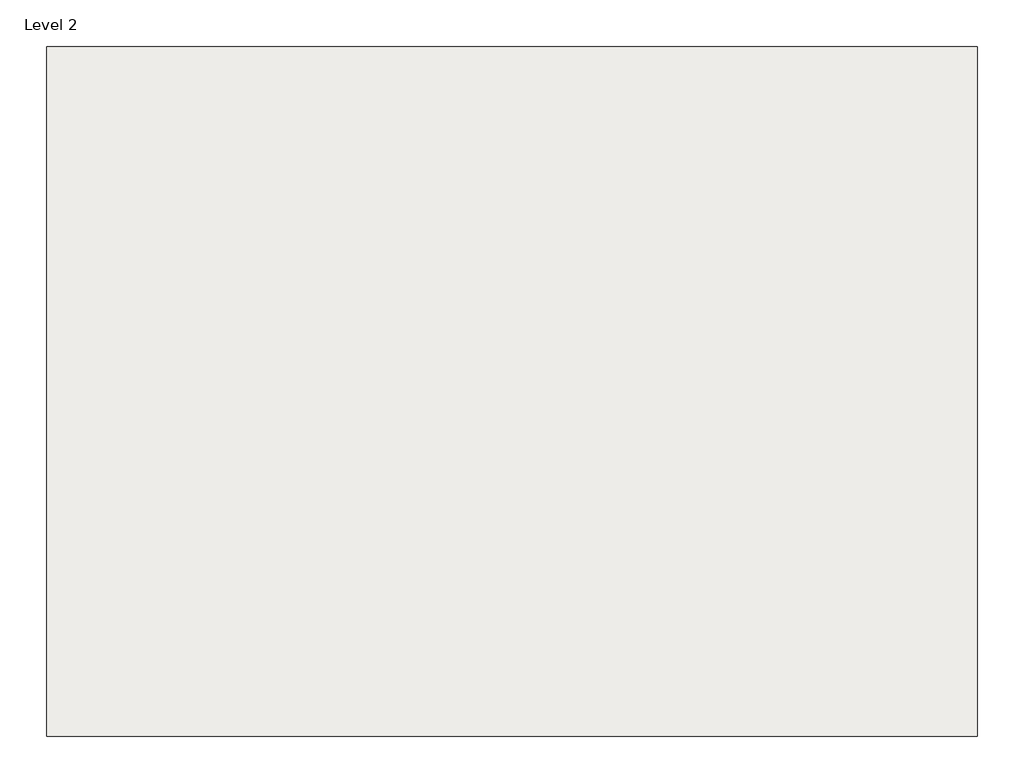
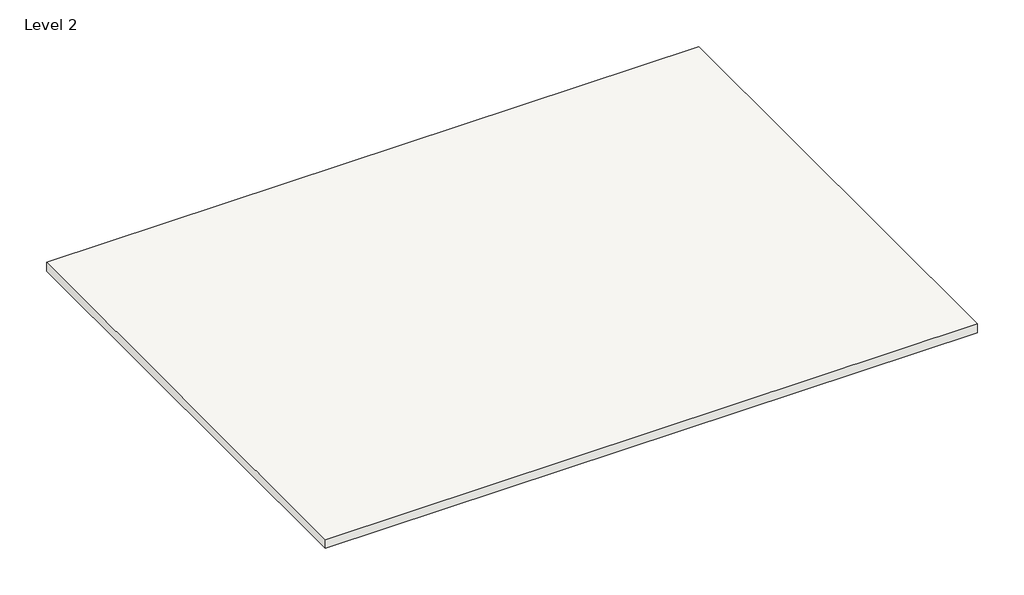
# One storey, incomplete: 1 roof.
"""IFC4 building model written with IfcOpenShell, lengths in millimetres."""

from ifc_helpers import new_model, si_unit, frame, origin, place, context, project, spatial, polyline, outline, extrude, element, save

model = new_model("IFC4")

# Units and contexts
model_context = context("Model", 3, world=origin())
ifc_project = project(units=[si_unit("LENGTHUNIT", "METRE", prefix="MILLI")], contexts=[model_context])

# Site, building, storey
site = spatial("IfcSite", under=ifc_project)
building = spatial("IfcBuilding", under=site)
storey = spatial("IfcBuildingStorey", under=building, Name="Level 2", Elevation=3048.0)

# Roof
placement = place(None, origin())
element("IfcRoof", 1, ObjectType="6\" floor", at=placement, inside=storey, context=model_context, shape_type="SweptSolid", body=[
    extrude(outline(polyline([(733.2620146, -5806.4506821), (-9858.5379854, -5806.4506821), (-9858.5379854, 2042.1493179), (733.2620146, 2042.1493179), (733.2620146, -5806.4506821)])), frame((0.0, 0.0, 3048.0), z_axis=(0.0, 0.0, 1.0), x_axis=(1.0, 0.0, 0.0)), (0.0, 0.0, 1.0), 152.4),
])

save(model, "model.ifc")

# Revit data of these elements
# Type "6\" floor"
#   Assembly Code = "B1020"
#   Layers, outside or top first: 0' - 6" no material (function 1)
# Element 1 (IfcRoof, "6\" floor")
#   built-in parameter 1001705 = 10.5 (stored number, unit not read)
#   built-in parameter 1001710 = 33615
#   Phase Created = New Construction
#   Materials on its faces: "Default Roof"
# Materials
#   "Default Roof": colour RGB 88 101 114, transparency 0, Cost = 0
